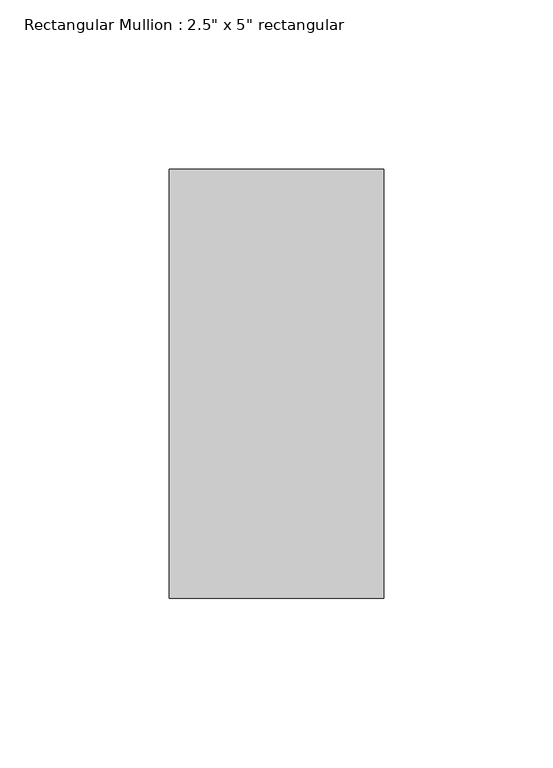
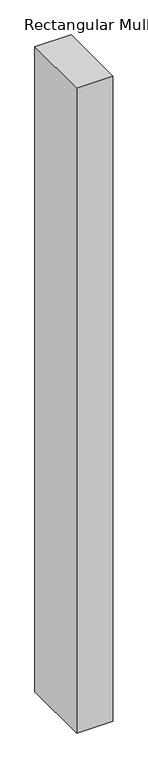
"""IFC4 building model written with IfcOpenShell, lengths in millimetres: member geometry."""

from ifc_helpers import new_model, si_unit, frame, origin, place, context, project, spatial, polyline, outline, extrude, source, transform, mapped, element, save


def member_9476229c(model_context):
    return source(origin(), model_context, "Body", "SweptSolid", [
        extrude(outline(polyline([(0.0, 63.5), (0.0, -63.5), (-63.5, -63.5), (-63.5, 63.5), (0.0, 63.5)])), frame((0.0, 0.0, -1195.0700002), z_axis=(0.0, 0.0, 1.0), x_axis=(1.0, 0.0, 0.0)), (0.0, 0.0, 1.0), 1195.0700002),
    ])


if __name__ == "__main__":
    model = new_model("IFC4")
    model_context = context("Model", 3, world=origin())
    ifc_project = project(units=[si_unit("LENGTHUNIT", "METRE", prefix="MILLI")], contexts=[model_context])
    site = spatial("IfcSite", under=ifc_project)
    building = spatial("IfcBuilding", under=site)
    placement = place(None, origin())
    member_shape = member_9476229c(model_context)
    element("IfcMember", 1, ObjectType="Rectangular Mullion : 2.5\" x 5\" rectangular", at=placement, inside=building, context=model_context, shape_type="MappedRepresentation", body=[
        mapped(member_shape, transform((0.0, 0.0, 0.0), x_axis=(1.0, 0.0, 0.0), y_axis=(0.0, 1.0, 0.0), z_axis=(0.0, 0.0, 1.0))),
    ])
    save(model, "model.ifc")

# Revit data of these elements
# Type "Rectangular Mullion : 2.5\" x 5\" rectangular"
#   built-in parameter 1007304 = 0.416667 (stored number, unit not read)
#   built-in parameter 1007301 = 0.104167 (stored number, unit not read)
#   built-in parameter 1007300 = 0.104167 (stored number, unit not read)
# Element 1 (IfcMember, "Rectangular Mullion : 2.5\" x 5\" rectangular")
#   Materials on its faces: "BLACK COLOUR"
# Materials
#   "BLACK COLOUR": class "Generic", colour RGB 120 120 120, transparency 0, Cost = 0
